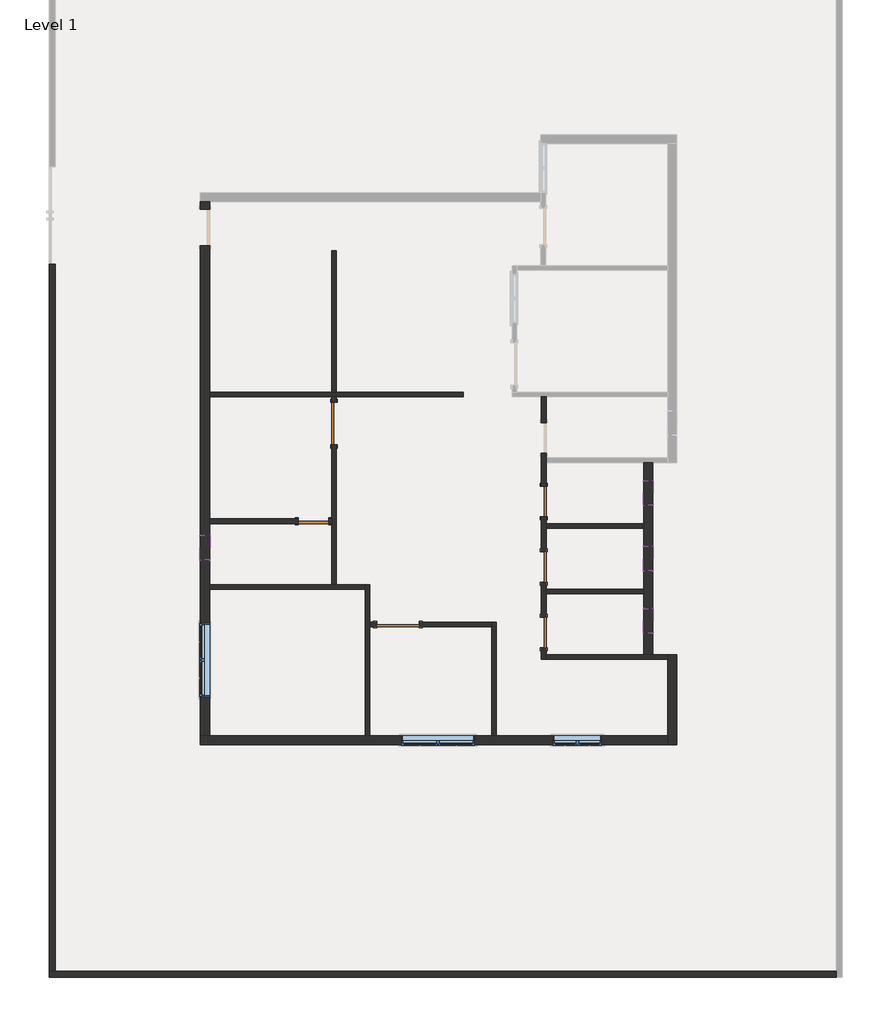
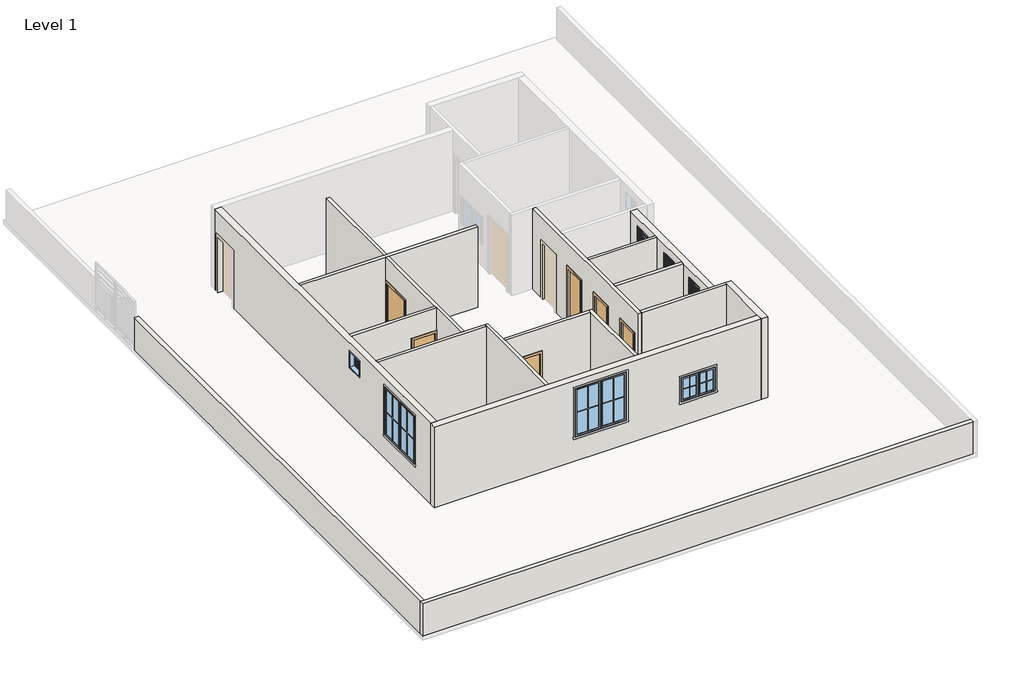
# One storey, part 1 of 2: 17 walls, 7 windows, 6 doors.
"""IFC4 building model written with IfcOpenShell, lengths in millimetres."""

from ifc_helpers import new_model, si_unit, frame, origin, origin_with_axes, place, context, project, spatial, polyline, outline, extrude, faceted_brep, transform, mapped, element, save
from components import door_78caadf7, door_214872d5, door_4c162e62, window_casement_double_win_4_c19c33cb, window_casement_double_win_6_ce442eab, window_f2d8fef0

model = new_model("IFC4")

# Units and contexts
model_context = context("Model", 3, world=origin())
ifc_project = project(units=[si_unit("LENGTHUNIT", "METRE", prefix="MILLI")], contexts=[model_context])

# Site, building, storey
site = spatial("IfcSite", under=ifc_project)
building = spatial("IfcBuilding", under=site)
storey = spatial("IfcBuildingStorey", under=building, Name="Level 1", Elevation=0.0)

# Doors
placement = place(None, origin())
door_shape = door_78caadf7(model_context)
element("IfcDoor", 1, ObjectType="Single-Flush : 2'6\"", at=placement, inside=storey, context=model_context, shape_type="MappedRepresentation", body=[
    mapped(door_shape, transform((-4241.833853, -925.804881, 0.0), x_axis=(1.0, 0.0, 0.0), y_axis=(0.0, 1.0, 0.0), z_axis=(0.0, 0.0, 1.0))),
])
door_2_shape = door_214872d5(model_context)
element("IfcDoor", 2, ObjectType="Single-Flush : 2'6\"", at=placement, inside=storey, context=model_context, shape_type="MappedRepresentation", body=[
    mapped(door_2_shape, transform((1511.266147, -430.504881, 0.0), x_axis=(0.0, -1.0, 0.0), y_axis=(1.0, 0.0, 0.0), z_axis=(0.0, 0.0, 1.0))),
])
element("IfcDoor", 3, ObjectType="Single-Flush : 2'6\"", at=placement, inside=storey, context=model_context, shape_type="MappedRepresentation", body=[
    mapped(door_2_shape, transform((1511.266147, -2068.804881, 0.0), x_axis=(0.0, -1.0, 0.0), y_axis=(1.0, 0.0, 0.0), z_axis=(0.0, 0.0, 1.0))),
])
element("IfcDoor", 4, ObjectType="Single-Flush : 2'6\"", at=placement, inside=storey, context=model_context, shape_type="MappedRepresentation", body=[
    mapped(door_2_shape, transform((1511.266147, -3707.104881, 0.0), x_axis=(0.0, -1.0, 0.0), y_axis=(1.0, 0.0, 0.0), z_axis=(0.0, 0.0, 1.0))),
])
door_3_shape = door_4c162e62(model_context)
element("IfcDoor", 5, ObjectType="Single-Flush : DOOR 3'6\"", at=placement, inside=storey, context=model_context, shape_type="MappedRepresentation", body=[
    mapped(door_3_shape, transform((-3733.833853, 1512.595119, 0.0), x_axis=(0.0, 1.0, 0.0), y_axis=(-1.0, 0.0, 0.0), z_axis=(0.0, 0.0, 1.0))),
])
element("IfcDoor", 6, ObjectType="Single-Flush : DOOR 3'6\"", at=placement, inside=storey, context=model_context, shape_type="MappedRepresentation", body=[
    mapped(door_3_shape, transform((-2133.633853, -3503.904881, 0.0), x_axis=(-1.0, 0.0, 0.0), y_axis=(0.0, -1.0, 0.0), z_axis=(0.0, 0.0, 1.0))),
])

# Walls
element("IfcWall", 7, ObjectType="CMD 6\"", at=placement, inside=storey, context=model_context, shape_type="Brep", body=[
    faceted_brep([(8818.8352257, -12170.1962844, 0.0), (-10688.3647743, -12170.1962844, 0.0), (-10840.7647743, -12170.1962844, 0.0), (-10840.7647743, -12170.1962844, 1219.2), (-10688.3647743, -12170.1962844, 1219.2), (8818.8352257, -12170.1962844, 1219.2), (8818.8352257, -12322.5962844, 0.0), (8818.8352257, -12322.5962844, 1219.2), (-10840.7647743, -12322.5962844, 1219.2), (-10840.7647743, -12322.5962844, 0.0)], [[[0, 1, 2, 3, 4, 5]], [[6, 7, 8, 9]], [[2, 1, 0, 6, 9]], [[5, 4, 3, 8, 7]], [[0, 5, 7, 6]], [[3, 2, 9, 8]]]),
])
element("IfcWall", 8, ObjectType="CMD 6\"", at=placement, inside=storey, context=model_context, shape_type="SweptSolid", body=[
    extrude(outline(polyline([(-10688.3647743, 5494.045119), (-10688.3647743, -12170.1962844), (-10840.7647743, -12170.1962844), (-10840.7647743, 5494.045119), (-10688.3647743, 5494.045119)])), origin_with_axes(), (0.0, 0.0, 1.0), 1219.2),
])
element("IfcWall", 9, ObjectType="WALL 4.5\"", at=placement, inside=storey, context=model_context, shape_type="Brep", body=[
    faceted_brep([(-6838.983853, 2179.345119, 0.0), (-3790.983853, 2179.345119, 0.0), (-3676.683853, 2179.345119, 0.0), (-501.683853, 2179.345119, 0.0), (-501.683853, 2179.345119, 3048.0), (-3676.683853, 2179.345119, 3048.0), (-3790.983853, 2179.345119, 3048.0), (-6838.983853, 2179.345119, 3048.0), (-6838.983853, 2293.645119, 0.0), (-6838.983853, 2293.645119, 3048.0), (-3790.983853, 2293.645119, 3048.0), (-3676.683853, 2293.645119, 3048.0), (-501.683853, 2293.645119, 3048.0), (-501.683853, 2293.645119, 0.0), (-3676.683853, 2293.645119, 0.0), (-3790.983853, 2293.645119, 0.0)], [[[0, 1, 2, 3, 4, 5, 6, 7]], [[8, 9, 10, 11, 12, 13, 14, 15]], [[3, 2, 1, 0, 8, 15, 14, 13]], [[4, 3, 13, 12]], [[0, 7, 9, 8]], [[7, 6, 5, 4, 12, 11, 10, 9]]]),
])
element("IfcWall", 10, ObjectType="WALL 4.5\"", at=placement, inside=storey, context=model_context, shape_type="Brep", body=[
    faceted_brep([(-2838.483853, -6278.854881, 0.0), (-2838.483853, -3561.054881, 0.0), (-2838.483853, -3446.754881, 0.0), (-2838.483853, -2506.954881, 0.0), (-2838.483853, -2506.954881, 3048.0), (-2838.483853, -3446.754881, 3048.0), (-2838.483853, -3561.054881, 3048.0), (-2838.483853, -6278.854881, 3048.0), (-2952.783853, -6278.854881, 0.0), (-2952.783853, -6278.854881, 3048.0), (-2952.783853, -2621.254881, 3048.0), (-2952.783853, -2506.954881, 3048.0), (-2952.783853, -2506.954881, 0.0), (-2952.783853, -2621.254881, 0.0)], [[[0, 1, 2, 3, 4, 5, 6, 7]], [[8, 9, 10, 11, 12, 13]], [[3, 2, 1, 0, 8, 13, 12]], [[0, 7, 9, 8]], [[4, 3, 12, 11]], [[7, 6, 5, 4, 11, 10, 9]]]),
])
element("IfcWall", 11, ObjectType="WALL 4.5\"", at=placement, inside=storey, context=model_context, shape_type="Brep", body=[
    faceted_brep([(-2952.783853, -2506.954881, 0.0), (-3676.683853, -2506.954881, 0.0), (-3790.983853, -2506.954881, 0.0), (-6838.983853, -2506.954881, 0.0), (-6838.983853, -2506.954881, 3048.0), (-3790.983853, -2506.954881, 3048.0), (-3676.683853, -2506.954881, 3048.0), (-2952.783853, -2506.954881, 3048.0), (-2952.783853, -2621.254881, 0.0), (-2952.783853, -2621.254881, 3048.0), (-6838.983853, -2621.254881, 3048.0), (-6838.983853, -2621.254881, 0.0)], [[[0, 1, 2, 3, 4, 5, 6, 7]], [[8, 9, 10, 11]], [[3, 2, 1, 0, 8, 11]], [[0, 7, 9, 8]], [[4, 3, 11, 10]], [[7, 6, 5, 4, 10, 9]]]),
])
element("IfcWall", 12, ObjectType="WALL 4.5\"", at=placement, inside=storey, context=model_context, shape_type="SweptSolid", body=[
    extrude(outline(polyline([(2133.6, -3860.833853), (0.0, -3860.833853), (0.0, -3790.983853), (3048.0, -3790.983853), (3048.0, -6838.983853), (0.0, -6838.983853), (0.0, -4622.833853), (2133.6, -4622.833853), (2133.6, -3860.833853)])), frame((0.0, -982.954881, 0.0), z_axis=(0.0, 1.0, 0.0), x_axis=(0.0, 0.0, 1.0)), (0.0, 0.0, 1.0), 114.3),
])
element("IfcWall", 13, ObjectType="WALL 4.5\"", at=placement, inside=storey, context=model_context, shape_type="Brep", body=[
    faceted_brep([(-3676.683853, 5836.945119, 0.0), (-3676.683853, 5836.945119, 3048.0), (-3676.683853, 2293.645119, 3048.0), (-3676.683853, 2293.645119, 0.0), (-3790.983853, 5836.945119, 3048.0), (-3790.983853, 5836.945119, 0.0), (-3790.983853, 2293.645119, 0.0), (-3790.983853, 2293.645119, 3048.0)], [[[0, 1, 2, 3]], [[4, 5, 6, 7]], [[5, 0, 3, 6]], [[1, 0, 5, 4]], [[3, 2, 7, 6]], [[1, 4, 7, 2]]]),
    faceted_brep([(-3676.683853, -2506.954881, 3048.0), (-3676.683853, -2506.954881, 0.0), (-3676.683853, 979.195119, 0.0), (-3676.683853, 979.195119, 2133.6), (-3676.683853, 2045.995119, 2133.6), (-3676.683853, 2045.995119, 0.0), (-3676.683853, 2179.345119, 0.0), (-3676.683853, 2179.345119, 3048.0), (-3790.983853, -2506.954881, 0.0), (-3790.983853, -2506.954881, 3048.0), (-3790.983853, -982.954881, 3048.0), (-3790.983853, -868.654881, 3048.0), (-3790.983853, 2179.345119, 3048.0), (-3790.983853, 2179.345119, 0.0), (-3790.983853, 2045.995119, 0.0), (-3790.983853, 2045.995119, 2133.6), (-3790.983853, 979.195119, 2133.6), (-3790.983853, 979.195119, 0.0), (-3790.983853, -868.654881, 0.0), (-3790.983853, -982.954881, 0.0)], [[[0, 1, 2, 3, 4, 5, 6, 7]], [[8, 9, 10, 11, 12, 13, 14, 15, 16, 17, 18, 19]], [[1, 8, 19, 18, 17, 2]], [[5, 14, 13, 6]], [[1, 0, 9, 8]], [[7, 6, 13, 12]], [[15, 14, 5, 4]], [[16, 15, 4, 3]], [[17, 16, 3, 2]], [[9, 0, 7, 12, 11, 10]]]),
])
element("IfcWall", 14, ObjectType="WALL 4.5\"", at=placement, inside=storey, context=model_context, shape_type="Brep", body=[
    faceted_brep([(1454.116147, -4088.104881, 2133.6), (1454.116147, -4088.104881, 0.0), (1454.116147, -4373.854881, 0.0), (1454.116147, -4373.854881, 3048.0), (1454.116147, 2179.345119, 3048.0), (1454.116147, 2179.345119, 0.0), (1454.116147, 1537.995119, 0.0), (1454.116147, 1537.995119, 2133.6), (1454.116147, 775.995119, 2133.6), (1454.116147, 775.995119, 0.0), (1454.116147, -49.504881, 0.0), (1454.116147, -49.504881, 2133.6), (1454.116147, -811.504881, 2133.6), (1454.116147, -811.504881, 0.0), (1454.116147, -1687.804881, 0.0), (1454.116147, -1687.804881, 2133.6), (1454.116147, -2449.804881, 2133.6), (1454.116147, -2449.804881, 0.0), (1454.116147, -3326.104881, 0.0), (1454.116147, -3326.104881, 2133.6), (1568.416147, -4373.854881, 0.0), (1568.416147, -4259.554881, 0.0), (1568.416147, -4088.104881, 0.0), (1568.416147, -4088.104881, 2133.6), (1568.416147, -3326.104881, 2133.6), (1568.416147, -3326.104881, 0.0), (1568.416147, -2735.554881, 0.0), (1568.416147, -2621.254881, 0.0), (1568.416147, -2449.804881, 0.0), (1568.416147, -2449.804881, 2133.6), (1568.416147, -1687.804881, 2133.6), (1568.416147, -1687.804881, 0.0), (1568.416147, -1097.254881, 0.0), (1568.416147, -982.954881, 0.0), (1568.416147, -811.504881, 0.0), (1568.416147, -811.504881, 2133.6), (1568.416147, -49.504881, 2133.6), (1568.416147, -49.504881, 0.0), (1568.416147, 541.045119, 0.0), (1568.416147, 655.345119, 0.0), (1568.416147, 775.995119, 0.0), (1568.416147, 775.995119, 2133.6), (1568.416147, 1537.995119, 2133.6), (1568.416147, 1537.995119, 0.0), (1568.416147, 2179.345119, 0.0), (1568.416147, 2179.345119, 3048.0), (1568.416147, 655.345119, 3048.0), (1568.416147, 541.045119, 3048.0), (1568.416147, -982.954881, 3048.0), (1568.416147, -1097.254881, 3048.0), (1568.416147, -2621.254881, 3048.0), (1568.416147, -2735.554881, 3048.0), (1568.416147, -4259.554881, 3048.0), (1568.416147, -4373.854881, 3048.0)], [[[0, 1, 2, 3, 4, 5, 6, 7, 8, 9, 10, 11, 12, 13, 14, 15, 16, 17, 18, 19]], [[20, 21, 22, 23, 24, 25, 26, 27, 28, 29, 30, 31, 32, 33, 34, 35, 36, 37, 38, 39, 40, 41, 42, 43, 44, 45, 46, 47, 48, 49, 50, 51, 52, 53]], [[6, 5, 44, 43]], [[10, 9, 40, 39, 38, 37]], [[14, 13, 34, 33, 32, 31]], [[18, 17, 28, 27, 26, 25]], [[2, 1, 22, 21, 20]], [[5, 4, 45, 44]], [[3, 2, 20, 53]], [[41, 40, 9, 8]], [[42, 41, 8, 7]], [[43, 42, 7, 6]], [[35, 34, 13, 12]], [[36, 35, 12, 11]], [[37, 36, 11, 10]], [[29, 28, 17, 16]], [[30, 29, 16, 15]], [[31, 30, 15, 14]], [[23, 22, 1, 0]], [[24, 23, 0, 19]], [[25, 24, 19, 18]], [[4, 3, 53, 52, 51, 50, 49, 48, 47, 46, 45]]]),
])
element("IfcWall", 15, ObjectType="WALL 4.5\"", at=placement, inside=storey, context=model_context, shape_type="Brep", body=[
    faceted_brep([(1568.416147, -4373.854881, 0.0), (4603.716147, -4373.854881, 0.0), (4603.716147, -4373.854881, 3048.0), (1568.416147, -4373.854881, 3048.0), (1568.416147, -4259.554881, 0.0), (1568.416147, -4259.554881, 3048.0), (4006.816147, -4259.554881, 3048.0), (4235.416147, -4259.554881, 3048.0), (4603.716147, -4259.554881, 3048.0), (4603.716147, -4259.554881, 0.0), (4235.416147, -4259.554881, 0.0), (4006.816147, -4259.554881, 0.0)], [[[0, 1, 2, 3]], [[4, 5, 6, 7, 8, 9, 10, 11]], [[1, 0, 4, 11, 10, 9]], [[0, 3, 5, 4]], [[2, 1, 9, 8]], [[3, 2, 8, 7, 6, 5]]]),
])
element("IfcWall", 16, ObjectType="WALL 4.5\"", at=placement, inside=storey, context=model_context, shape_type="SweptSolid", body=[
    extrude(outline(polyline([(4006.816147, -2735.554881), (1568.416147, -2735.554881), (1568.416147, -2621.254881), (4006.816147, -2621.254881), (4006.816147, -2735.554881)])), origin_with_axes(), (0.0, 0.0, 1.0), 3048.0),
])
element("IfcWall", 17, ObjectType="WALL 4.5\"", at=placement, inside=storey, context=model_context, shape_type="SweptSolid", body=[
    extrude(outline(polyline([(4006.816147, -1097.254881), (1568.416147, -1097.254881), (1568.416147, -982.954881), (4006.816147, -982.954881), (4006.816147, -1097.254881)])), origin_with_axes(), (0.0, 0.0, 1.0), 3048.0),
])
element("IfcWall", 18, ObjectType="WALL 4.5\"", at=placement, inside=storey, context=model_context, shape_type="Brep", body=[
    faceted_brep([(323.816147, -6278.854881, 0.0), (323.816147, -3446.754881, 0.0), (323.816147, -3446.754881, 3048.0), (323.816147, -6278.854881, 3048.0), (209.516147, -6278.854881, 0.0), (209.516147, -6278.854881, 3048.0), (209.516147, -3561.054881, 3048.0), (209.516147, -3446.754881, 3048.0), (209.516147, -3446.754881, 0.0), (209.516147, -3561.054881, 0.0)], [[[0, 1, 2, 3]], [[4, 5, 6, 7, 8, 9]], [[1, 0, 4, 9, 8]], [[0, 3, 5, 4]], [[2, 1, 8, 7]], [[3, 2, 7, 6, 5]]]),
])
element("IfcWall", 19, ObjectType="WALL 4.5\"", at=placement, inside=storey, context=model_context, shape_type="SweptSolid", body=[
    extrude(outline(polyline([(0.0, -2838.483853), (0.0, -2667.033853), (2133.6, -2667.033853), (2133.6, -1600.233853), (0.0, -1600.233853), (0.0, 209.516147), (3048.0, 209.516147), (3048.0, -2838.483853), (0.0, -2838.483853)])), frame((0.0, -3561.054881, 0.0), z_axis=(0.0, 1.0, 0.0), x_axis=(0.0, 0.0, 1.0)), (0.0, 0.0, 1.0), 114.3),
])
element("IfcWall", 20, ObjectType="WALL 9\"", at=placement, inside=storey, context=model_context, shape_type="Brep", body=[
    faceted_brep([(4006.816147, 541.045119, 0.0), (4006.816147, -982.954881, 0.0), (4006.816147, -1097.254881, 0.0), (4006.816147, -2621.254881, 0.0), (4006.816147, -2735.554881, 0.0), (4006.816147, -4259.554881, 0.0), (4006.816147, -4259.554881, 3048.0), (4006.816147, -2735.554881, 3048.0), (4006.816147, -2621.254881, 3048.0), (4006.816147, -1097.254881, 3048.0), (4006.816147, -982.954881, 3048.0), (4006.816147, 541.045119, 3048.0), (4006.816147, -525.754881, 2743.2), (4006.816147, -525.754881, 2133.6), (4006.816147, 83.845119, 2133.6), (4006.816147, 83.845119, 2743.2), (4006.816147, -2164.054881, 2743.2), (4006.816147, -2164.054881, 2133.6), (4006.816147, -1554.454881, 2133.6), (4006.816147, -1554.454881, 2743.2), (4006.816147, -3719.804881, 2743.2), (4006.816147, -3719.804881, 2133.6), (4006.816147, -3110.204881, 2133.6), (4006.816147, -3110.204881, 2743.2), (4235.416147, 541.045119, 0.0), (4235.416147, 541.045119, 3048.0), (4235.416147, -4259.554881, 3048.0), (4235.416147, -4259.554881, 0.0), (4235.416147, -525.754881, 2743.2), (4235.416147, 83.845119, 2743.2), (4235.416147, 83.845119, 2133.6), (4235.416147, -525.754881, 2133.6), (4235.416147, -2164.054881, 2743.2), (4235.416147, -1554.454881, 2743.2), (4235.416147, -1554.454881, 2133.6), (4235.416147, -2164.054881, 2133.6), (4235.416147, -3719.804881, 2743.2), (4235.416147, -3110.204881, 2743.2), (4235.416147, -3110.204881, 2133.6), (4235.416147, -3719.804881, 2133.6)], [[[0, 1, 2, 3, 4, 5, 6, 7, 8, 9, 10, 11], [12, 13, 14, 15], [16, 17, 18, 19], [20, 21, 22, 23]], [[24, 25, 26, 27], [28, 29, 30, 31], [32, 33, 34, 35], [36, 37, 38, 39]], [[5, 4, 3, 2, 1, 0, 24, 27]], [[0, 11, 25, 24]], [[6, 5, 27, 26]], [[13, 12, 28, 31]], [[14, 13, 31, 30]], [[15, 14, 30, 29]], [[12, 15, 29, 28]], [[17, 16, 32, 35]], [[18, 17, 35, 34]], [[19, 18, 34, 33]], [[16, 19, 33, 32]], [[21, 20, 36, 39]], [[22, 21, 39, 38]], [[23, 22, 38, 37]], [[20, 23, 37, 36]], [[11, 10, 9, 8, 7, 6, 26, 25]]]),
])
element("IfcWall", 21, ObjectType="WALL 9\"", at=placement, inside=storey, context=model_context, shape_type="Brep", body=[
    faceted_brep([(4603.716147, -4259.554881, 0.0), (4603.716147, -4373.854881, 0.0), (4603.716147, -6278.854881, 0.0), (4603.716147, -6507.454881, 0.0), (4603.716147, -6507.454881, 3048.0), (4603.716147, -6278.854881, 3048.0), (4603.716147, -4373.854881, 3048.0), (4603.716147, -4259.554881, 3048.0), (4832.316147, -4259.554881, 0.0), (4832.316147, -4259.554881, 3048.0), (4832.316147, -6507.454881, 3048.0), (4832.316147, -6507.454881, 0.0)], [[[0, 1, 2, 3, 4, 5, 6, 7]], [[8, 9, 10, 11]], [[3, 2, 1, 0, 8, 11]], [[4, 3, 11, 10]], [[0, 7, 9, 8]], [[7, 6, 5, 4, 10, 9]]]),
])
element("IfcWall", 22, ObjectType="WALL 9\"", at=placement, inside=storey, context=model_context, shape_type="Brep", body=[
    faceted_brep([(4603.716147, -6278.854881, 0.0), (323.816147, -6278.854881, 0.0), (209.516147, -6278.854881, 0.0), (-2838.483853, -6278.854881, 0.0), (-2952.783853, -6278.854881, 0.0), (-6838.983853, -6278.854881, 0.0), (-7067.583853, -6278.854881, 0.0), (-7067.583853, -6278.854881, 3048.0), (-6838.983853, -6278.854881, 3048.0), (-2952.783853, -6278.854881, 3048.0), (-2838.483853, -6278.854881, 3048.0), (209.516147, -6278.854881, 3048.0), (323.816147, -6278.854881, 3048.0), (4603.716147, -6278.854881, 3048.0), (-2044.733853, -6278.854881, 2743.2), (-2044.733853, -6278.854881, 914.4), (-215.933853, -6278.854881, 914.4), (-215.933853, -6278.854881, 2743.2), (1739.866147, -6278.854881, 1828.8), (1739.866147, -6278.854881, 914.4), (2959.066147, -6278.854881, 914.4), (2959.066147, -6278.854881, 1828.8), (4603.716147, -6507.454881, 0.0), (4603.716147, -6507.454881, 3048.0), (-7067.583853, -6507.454881, 3048.0), (-7067.583853, -6507.454881, 0.0), (-2044.733853, -6507.454881, 2743.2), (-215.933853, -6507.454881, 2743.2), (-215.933853, -6507.454881, 914.4), (-2044.733853, -6507.454881, 914.4), (1739.866147, -6507.454881, 1828.8), (2959.066147, -6507.454881, 1828.8), (2959.066147, -6507.454881, 914.4), (1739.866147, -6507.454881, 914.4)], [[[0, 1, 2, 3, 4, 5, 6, 7, 8, 9, 10, 11, 12, 13], [14, 15, 16, 17], [18, 19, 20, 21]], [[22, 23, 24, 25], [26, 27, 28, 29], [30, 31, 32, 33]], [[6, 5, 4, 3, 2, 1, 0, 22, 25]], [[0, 13, 23, 22]], [[7, 6, 25, 24]], [[15, 14, 26, 29]], [[16, 15, 29, 28]], [[17, 16, 28, 27]], [[14, 17, 27, 26]], [[19, 18, 30, 33]], [[20, 19, 33, 32]], [[21, 20, 32, 31]], [[18, 21, 31, 30]], [[13, 12, 11, 10, 9, 8, 7, 24, 23]]]),
])
element("IfcWall", 23, ObjectType="WALL 9\"", at=placement, inside=storey, context=model_context, shape_type="Brep", body=[
    faceted_brep([(-6838.983853, 6865.645119, 2133.6), (-6838.983853, 6865.645119, 0.0), (-6838.983853, 7056.145119, 0.0), (-6838.983853, 7056.145119, 3048.0), (-6838.983853, 2293.645119, 3048.0), (-6838.983853, 2179.345119, 3048.0), (-6838.983853, -868.654881, 3048.0), (-6838.983853, -982.954881, 3048.0), (-6838.983853, -2506.954881, 3048.0), (-6838.983853, -2621.254881, 3048.0), (-6838.983853, -6278.854881, 3048.0), (-6838.983853, -6278.854881, 0.0), (-6838.983853, -2621.254881, 0.0), (-6838.983853, -2506.954881, 0.0), (-6838.983853, -982.954881, 0.0), (-6838.983853, -868.654881, 0.0), (-6838.983853, 2179.345119, 0.0), (-6838.983853, 2293.645119, 0.0), (-6838.983853, 5951.245119, 0.0), (-6838.983853, 5951.245119, 2133.6), (-6838.983853, -3478.504881, 2743.2), (-6838.983853, -3478.504881, 914.4), (-6838.983853, -5307.304881, 914.4), (-6838.983853, -5307.304881, 2743.2), (-6838.983853, -1281.404881, 2743.2), (-6838.983853, -1281.404881, 2133.6), (-6838.983853, -1891.004881, 2133.6), (-6838.983853, -1891.004881, 2743.2), (-7067.583853, 7056.145119, 0.0), (-7067.583853, 6865.645119, 0.0), (-7067.583853, 6865.645119, 2133.6), (-7067.583853, 5951.245119, 2133.6), (-7067.583853, 5951.245119, 0.0), (-7067.583853, -6278.854881, 0.0), (-7067.583853, -6278.854881, 3048.0), (-7067.583853, 7056.145119, 3048.0), (-7067.583853, -3478.504881, 2743.2), (-7067.583853, -5307.304881, 2743.2), (-7067.583853, -5307.304881, 914.4), (-7067.583853, -3478.504881, 914.4), (-7067.583853, -1281.404881, 2743.2), (-7067.583853, -1891.004881, 2743.2), (-7067.583853, -1891.004881, 2133.6), (-7067.583853, -1281.404881, 2133.6)], [[[0, 1, 2, 3, 4, 5, 6, 7, 8, 9, 10, 11, 12, 13, 14, 15, 16, 17, 18, 19], [20, 21, 22, 23], [24, 25, 26, 27]], [[28, 29, 30, 31, 32, 33, 34, 35], [36, 37, 38, 39], [40, 41, 42, 43]], [[2, 1, 29, 28]], [[18, 17, 16, 15, 14, 13, 12, 11, 33, 32]], [[11, 10, 34, 33]], [[3, 2, 28, 35]], [[21, 20, 36, 39]], [[22, 21, 39, 38]], [[23, 22, 38, 37]], [[20, 23, 37, 36]], [[25, 24, 40, 43]], [[26, 25, 43, 42]], [[27, 26, 42, 41]], [[24, 27, 41, 40]], [[30, 29, 1, 0]], [[31, 30, 0, 19]], [[32, 31, 19, 18]], [[10, 9, 8, 7, 6, 5, 4, 3, 35, 34]]]),
])

# Windows
window_casement_double_win_4_shape = window_casement_double_win_4_c19c33cb(model_context)
element("IfcWindow", 24, ObjectType="Window-Casement-Double : WIN 4'", at=placement, inside=storey, context=model_context, shape_type="MappedRepresentation", body=[
    mapped(window_casement_double_win_4_shape, transform((2349.466147, -6393.154881, 0.0), x_axis=(-1.0, 0.0, 0.0), y_axis=(0.0, -1.0, 0.0), z_axis=(0.0, 0.0, 1.0))),
])
window_casement_double_win_6_shape = window_casement_double_win_6_ce442eab(model_context)
element("IfcWindow", 25, ObjectType="Window-Casement-Double : WIN 6'", at=placement, inside=storey, context=model_context, shape_type="MappedRepresentation", body=[
    mapped(window_casement_double_win_6_shape, transform((-6953.283853, -4392.904881, 0.0), x_axis=(0.0, 1.0, 0.0), y_axis=(-1.0, 0.0, 0.0), z_axis=(0.0, 0.0, 1.0))),
])
element("IfcWindow", 26, ObjectType="Window-Casement-Double : WIN 6'", at=placement, inside=storey, context=model_context, shape_type="MappedRepresentation", body=[
    mapped(window_casement_double_win_6_shape, transform((-1130.333853, -6393.154881, 0.0), x_axis=(-1.0, 0.0, 0.0), y_axis=(0.0, -1.0, 0.0), z_axis=(0.0, 0.0, 1.0))),
])
window_shape = window_f2d8fef0(model_context)
element("IfcWindow", 27, ObjectType="Window-Louvers : 24\" x 24\"", at=placement, inside=storey, context=model_context, shape_type="MappedRepresentation", body=[
    mapped(window_shape, transform((4114.766147, -220.954881, 1219.2), x_axis=(0.0, 1.0, 0.0), y_axis=(-1.0, 0.0, 0.0), z_axis=(0.0, 0.0, 1.0))),
])
element("IfcWindow", 28, ObjectType="Window-Louvers : 24\" x 24\"", at=placement, inside=storey, context=model_context, shape_type="MappedRepresentation", body=[
    mapped(window_shape, transform((4114.766147, -1859.254881, 1219.2), x_axis=(0.0, 1.0, 0.0), y_axis=(-1.0, 0.0, 0.0), z_axis=(0.0, 0.0, 1.0))),
])
element("IfcWindow", 29, ObjectType="Window-Louvers : 24\" x 24\"", at=placement, inside=storey, context=model_context, shape_type="MappedRepresentation", body=[
    mapped(window_shape, transform((4114.766147, -3415.004881, 1219.2), x_axis=(0.0, 1.0, 0.0), y_axis=(-1.0, 0.0, 0.0), z_axis=(0.0, 0.0, 1.0))),
])
element("IfcWindow", 30, ObjectType="Window-Louvers : 24\" x 24\"", at=placement, inside=storey, context=model_context, shape_type="MappedRepresentation", body=[
    mapped(window_shape, transform((-6946.933853, -1586.204881, 1219.2), x_axis=(0.0, -1.0, 0.0), y_axis=(1.0, 0.0, 0.0), z_axis=(0.0, 0.0, 1.0))),
])

save(model, "model.ifc")

# Revit data of these elements
# Type "Single-Flush : 2'6\""
#   Type Mark = "10"
#   Construction Type Id = "MDOOR"
#   Assembly Code = "C1020"
#   Analytic Construction = "Metal"
#   Thickness = 0' - 2"
#   Heat Transfer Coefficient (U) = 0.651978 BTU/(h·ft²·°F)
#   Height = 7' - 0"
#   Trim Projection Ext = 0' - 1"
#   Trim Projection Int = 0' - 1"
#   Trim Width = 0' - 3"
#   Width = 2' - 6"
#   Define Thermal Properties by = 1
#   Door Material = Door - Panel
#   Frame Material = Door - Frame
#   Visual Light Transmittance = 0
#   Solar Heat Gain Coefficient = 0
#   Function = (empty or 0)
#   Wall Closure = (empty or 0)
# Type "Single-Flush : DOOR 3'6\""
#   Type Mark = "9"
#   Construction Type Id = "MDOOR"
#   Assembly Code = "C1020"
#   Analytic Construction = "Metal"
#   Thickness = 0' - 2"
#   Heat Transfer Coefficient (U) = 0.651978 BTU/(h·ft²·°F)
#   Height = 7' - 0"
#   Trim Projection Ext = 0' - 1"
#   Trim Projection Int = 0' - 1"
#   Trim Width = 0' - 3"
#   Width = 3' - 6"
#   Define Thermal Properties by = 1
#   Door Material = Door - Panel
#   Frame Material = Door - Frame
#   Visual Light Transmittance = 0
#   Solar Heat Gain Coefficient = 0
#   Function = (empty or 0)
#   Wall Closure = (empty or 0)
# Type "CMD 6\""
#   Assembly Code = "B2010"
#   Layers, outside or top first: 0' - 6" no material (function 1)
# Type "WALL 4.5\""
#   Assembly Code = "B2010"
#   Layers, outside or top first: 0' - 4 1/2" no material (function 1)
# Type "WALL 9\""
#   Assembly Code = "B2010"
#   Layers, outside or top first: 0' - 9" no material (function 1)
# Type "Window-Casement-Double : WIN 4'"
#   Type Mark = "18"
#   Fire Rating = "0.5h"
#   Assembly Code = "B2020100"
#   Analytic Construction = "Double glazing - domestic"
#   Frame Extension [instance default] = 0' - 0 1/4"
#   Window Inset [instance default] = 0' - 0"
#   Wall Thickness [instance default] = 0' - 6"
#   Interior Wall Closure [instance default] = 0' - 2 1/4"
#   Half Width = 2' - 0"
#   Visual Light Transmittance = 0.81
#   Thermal Resistance (R) = 1.8146 (h·ft²·°F)/BTU
#   Solar Heat Gain Coefficient = 0.76
#   Rough Width = 4' - 0 1/2"
#   Rough Height = 3' - 0 1/2"
#   Height = 3' - 0"
#   Heat Transfer Coefficient (U) = 0.5511 BTU/(h·ft²·°F)
#   Exterior Wall Closure [instance default] = 0' - 1 1/4"
#   Extension Jamb [instance default] = 0' - 2 1/4"
#   Default Sill Height = 3' - 0"
#   Width = 4' - 0"
#   Muntin Visibility = yes
#   Interior Trim Visibility [instance default] = yes
#   Exterior Trim Visibility [instance default] = yes
#   Extension Jamb Visibility [instance default] = yes
#   Interior Trim Material = Wood - Stained
#   Muntin Pattern = Muntin Pattern_2x2 : Muntin Pattern_2x2
#   Interior Trim = Trim-Window-Interior-Flat : Picture Frame
#   Interior Frame Material = Wood - Stained
#   Glass Panel Material = Glass
#   Exterior Trim Material = Clad - White
#   Exterior Trim = Trim-Window-Exterior-Flat : with Sill
#   Exterior Frame Material = Clad - White
#   Wall Closure = (empty or 0)
# Type "Window-Casement-Double : WIN 6'"
#   Type Mark = "19"
#   Fire Rating = "0.5h"
#   Assembly Code = "B2020100"
#   Analytic Construction = "Double glazing - domestic"
#   Frame Extension [instance default] = 0' - 0 1/4"
#   Window Inset [instance default] = 0' - 0"
#   Wall Thickness [instance default] = 0' - 6"
#   Interior Wall Closure [instance default] = 0' - 2 1/4"
#   Half Width = 3' - 0"
#   Visual Light Transmittance = 0.81
#   Thermal Resistance (R) = 1.8146 (h·ft²·°F)/BTU
#   Solar Heat Gain Coefficient = 0.76
#   Rough Width = 6' - 0 1/2"
#   Rough Height = 6' - 0 1/2"
#   Height = 6' - 0"
#   Heat Transfer Coefficient (U) = 0.5511 BTU/(h·ft²·°F)
#   Exterior Wall Closure [instance default] = 0' - 1 1/4"
#   Extension Jamb [instance default] = 0' - 2 1/4"
#   Default Sill Height = 3' - 0"
#   Width = 6' - 0"
#   Muntin Visibility = yes
#   Interior Trim Visibility [instance default] = yes
#   Exterior Trim Visibility [instance default] = yes
#   Extension Jamb Visibility [instance default] = yes
#   Interior Trim Material = Wood - Stained
#   Muntin Pattern = Muntin Pattern_2x2 : Muntin Pattern_2x2
#   Interior Trim = Trim-Window-Interior-Flat : Picture Frame
#   Interior Frame Material = Wood - Stained
#   Glass Panel Material = Glass
#   Exterior Trim Material = Clad - White
#   Exterior Trim = Trim-Window-Exterior-Flat : with Sill
#   Exterior Frame Material = Clad - White
#   Wall Closure = (empty or 0)
# Type "Window-Louvers : 24\" x 24\""
#   Type Mark = "20"
#   Construction Type Id = "GSP4R"
#   Assembly Code = "B20"
#   Analytic Construction = "1/8 in Pilkington single glazing"
#   Visual Light Transmittance = 0.9
#   Thermal Resistance (R) = 1.53941 (h·ft²·°F)/BTU
#   Solar Heat Gain Coefficient = 0.78
#   Max Height = 1' - 11.74264"
#   Height = 2' - 0"
#   Heat Transfer Coefficient (U) = 0.6496 BTU/(h·ft²·°F)
#   Blade Width [instance default] = 1' - 10 1/2"
#   Blade Vertical Thickness = 0' - 0.35355"
#   Blade Thickness = 0' - 0 1/4"
#   Blade Spacing = 0' - 1 1/2"
#   Blade Height = 0' - 1.85355"
#   Blade Depth = 0' - 3"
#   Blade Angle = 45.00°
#   Default Sill Height = 3' - 0"
#   Trim Projection_Exterior = 0' - 0 1/2"
#   Trim Projection_Interior = 0' - 0 1/2"
#   Trim Width_Exterior = 0' - 1 1/2"
#   Trim Width_Interior = 0' - 1 1/2"
#   Width = 2' - 0"
#   Max Blade Count = 12
#   Define Thermal Properties by = 1
#   Blade Count = 12
#   Frame Material = Birch
#   Louver Material = Birch
#   Trim Exterior Material = Birch
#   Trim Interior Material = Birch
#   Wall Closure = (empty or 0)
# Elements 1, 2, 3, 4 (IfcDoor, "Single-Flush : 2'6\"")
#   Phase Created = New Construction
#   Materials on its faces: "Door - Frame", "Door - Panel"
# Elements 5, 6 (IfcDoor, "Single-Flush : DOOR 3'6\"")
#   Phase Created = New Construction
#   Materials on its faces: "Door - Frame", "Door - Panel"
# Elements 7, 8 (IfcWall, "CMD 6\"")
#   Top Offset = 0' - 0"
#   Base Offset = 0' - 0"
#   Unconnected Height = 4' - 0"
#   wall height = 4' - 0"
#   Phase Created = New Construction
#   Base Constraint = Level 1
#   Materials on its faces: "Default Wall", "Clad - White", "Cherry"
# Elements 9, 10, 11, 12, 13, 14, 15, 16, 17, 18, 19 (IfcWall, "WALL 4.5\"")
#   Top Offset = 0' - 0"
#   Base Offset = 0' - 0"
#   Unconnected Height = 10' - 0"
#   wall height = 10' - 0"
#   Phase Created = New Construction
#   Base Constraint = Level 1
#   Materials on its faces: "Default Wall"
# Elements 20, 21, 22, 23 (IfcWall, "WALL 9\"")
#   Top Offset = 0' - 0"
#   Base Offset = 0' - 0"
#   Unconnected Height = 10' - 0"
#   wall height = 10' - 0"
#   Phase Created = New Construction
#   Base Constraint = Level 1
#   Materials on its faces: "Default Wall", "Wood - Stained"
# Element 24 (IfcWindow, "Window-Casement-Double : WIN 4'")
#   Mark = "3"
#   Window Inset = 0' - 0"
#   Interior Wall Closure = 0' - 2 1/4"
#   Frame Extension = 0' - 0 1/4"
#   Exterior Wall Closure = 0' - 1 1/4"
#   Interior Trim Visibility = yes
#   Exterior Trim Visibility = yes
#   Phase Created = New Construction
#   Materials on its faces: "Wood - Stained", "Glass", "Clad - White"
# Element 25 (IfcWindow, "Window-Casement-Double : WIN 6'")
#   Mark = "1"
#   Window Inset = 0' - 0"
#   Interior Wall Closure = 0' - 2 1/4"
#   Frame Extension = 0' - 0 1/4"
#   Exterior Wall Closure = 0' - 1 1/4"
#   Interior Trim Visibility = yes
#   Exterior Trim Visibility = yes
#   Phase Created = New Construction
#   Materials on its faces: "Wood - Stained", "Glass", "Clad - White"
# Element 26 (IfcWindow, "Window-Casement-Double : WIN 6'")
#   Mark = "2"
#   Window Inset = 0' - 0"
#   Interior Wall Closure = 0' - 2 1/4"
#   Frame Extension = 0' - 0 1/4"
#   Exterior Wall Closure = 0' - 1 1/4"
#   Interior Trim Visibility = yes
#   Exterior Trim Visibility = yes
#   Phase Created = New Construction
#   Materials on its faces: "Wood - Stained", "Glass", "Clad - White"
# Element 27 (IfcWindow, "Window-Louvers : 24\" x 24\"")
#   Mark = "7"
#   Blade Width = 1' - 10 1/2"
#   Phase Created = New Construction
#   Materials on its faces: "Birch"
# Element 28 (IfcWindow, "Window-Louvers : 24\" x 24\"")
#   Mark = "8"
#   Blade Width = 1' - 10 1/2"
#   Phase Created = New Construction
#   Materials on its faces: "Birch"
# Element 29 (IfcWindow, "Window-Louvers : 24\" x 24\"")
#   Mark = "9"
#   Blade Width = 1' - 10 1/2"
#   Phase Created = New Construction
#   Materials on its faces: "Birch"
# Element 30 (IfcWindow, "Window-Louvers : 24\" x 24\"")
#   Mark = "10"
#   Blade Width = 1' - 10 1/2"
#   Phase Created = New Construction
#   Materials on its faces: "Birch"
# Materials
#   "Door - Panel": class "Wood", colour RGB 210 159 95, transparency 0, Cost = 0
#   "Door - Frame": colour RGB 118 70 51, transparency 0, Cost = 0
#   "Wood - Stained": class "Wood", colour RGB 224 178 126, transparency 0, Cost = 0
#   "Glass": class "Glass", colour RGB 0 128 192, transparency 0.75, Description = "Soda Lime Glass", Cost = 0
#   "Clad - White": class "Wood", colour RGB 242 242 238, transparency 0, Cost = 0
#   "Birch": class "Wood", colour RGB 224 178 126, transparency 0, Description = "Betula Alleghaniensis", Cost = 0
#   "Default Wall": colour RGB 128 128 128, transparency 0, Cost = 0
#   "Cherry": class "Wood", colour RGB 226 177 128, transparency 0, Description = "Prunus Serotina", Cost = 0
